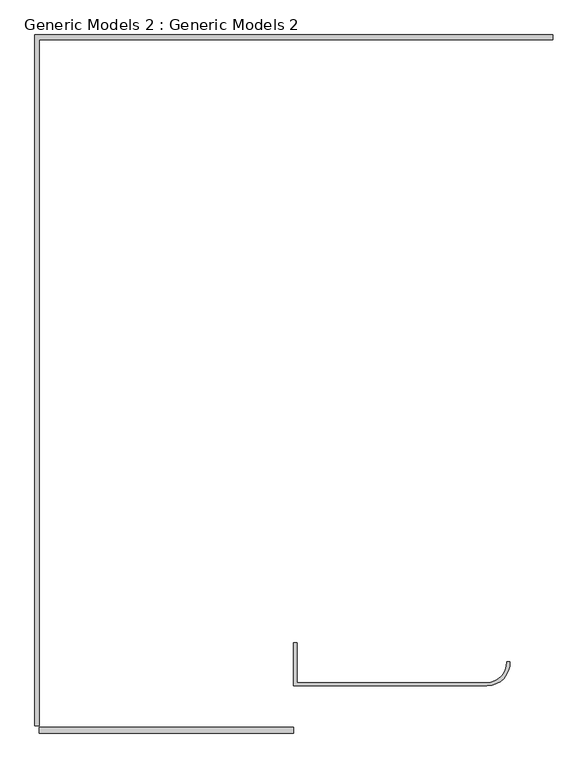
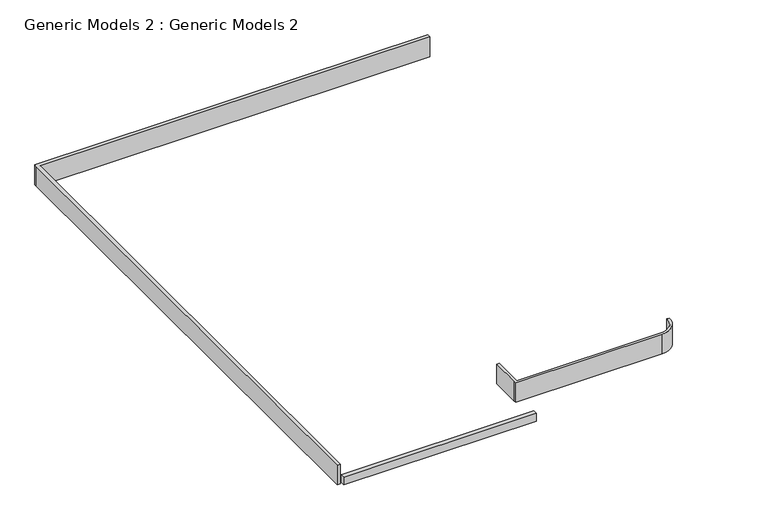
"""IFC4 building model written with IfcOpenShell, lengths in millimetres: proxy geometry, Generic Models 2 : Generic Models 2."""

from ifc_helpers import new_model, si_unit, point, frame, frame_2d, origin, origin_with_axes, place, context, project, spatial, polyline, circle_curve, trimmed, segment, composite_curve, outline, extrude, source, transform, mapped, element, save


def generic_models_2_generic_models_2_74674079(model_context):
    return source(origin(), model_context, "Body", "SweptSolid", [
        extrude(outline(polyline([(-42650.6472522, 6250.4436329), (-42650.6472522, 6059.9436329), (-51134.2472522, 6059.9436329), (-51134.2472522, 6250.4436329), (-42650.6472522, 6250.4436329)])), frame((0.0, 0.0, 91.4796875), z_axis=(0.0, 0.0, 1.0), x_axis=(1.0, 0.0, 0.0)), (0.0, 0.0, 1.0), 358.4773438),
        extrude(outline(polyline([(-33990.9791975, 29336.6093243), (-33990.9791975, 29177.2755965), (-51132.7755215, 29177.2755965), (-51132.7755215, 6297.7565956), (-51278.13478, 6297.7565956), (-51278.13478, 29257.5093141), (-51278.13478, 29336.6093243), (-33990.9791975, 29336.6093243)])), origin_with_axes(), (0.0, 0.0, 1.0), 914.4),
        extrude(outline(composite_curve([segment(trimmed(circle_curve(frame_2d((-36189.4383946, 8397.9312492)), 652.3904346), [point((-36189.4383946, 7745.5408146))], [point((-35538.4124894, 8440.1041063))], True, "CARTESIAN"), True, "CONTINUOUS"), segment(polyline([(-35538.4124894, 8440.1041063), (-35423.3146623, 8440.1041063)]), True, "CONTINUOUS"), segment(trimmed(circle_curve(frame_2d((-36189.4383946, 8410.6312492)), 766.6904346), [point((-35423.3146623, 8440.1041063))], [point((-36189.4383946, 7643.9408146))], False, "CARTESIAN"), True, "CONTINUOUS"), segment(polyline([(-36189.4383946, 7643.9408146), (-42641.0383946, 7643.9408146), (-42641.0383946, 7745.5408146), (-42641.0383946, 9075.1041063), (-42534.6852357, 9075.1041063), (-42534.6852357, 7745.5408146), (-36189.4383946, 7745.5408146)]), True, "CONTINUOUS")], self_intersect=False)), origin_with_axes(), (0.0, 0.0, 1.0), 914.4),
    ])


if __name__ == "__main__":
    model = new_model("IFC4")
    model_context = context("Model", 3, world=origin())
    ifc_project = project(units=[si_unit("LENGTHUNIT", "METRE", prefix="MILLI")], contexts=[model_context])
    site = spatial("IfcSite", under=ifc_project)
    building = spatial("IfcBuilding", under=site)
    placement = place(None, origin())
    generic_models_2_generic_models_2_shape = generic_models_2_generic_models_2_74674079(model_context)
    element("IfcBuildingElementProxy", 1, Name="Generic Models 2 : Generic Models 2", ObjectType="Generic Models 2 : Generic Models 2", at=placement, inside=building, context=model_context, shape_type="MappedRepresentation", body=[
        mapped(generic_models_2_generic_models_2_shape, transform((0.0, 0.0, 0.0), x_axis=(1.0, 0.0, 0.0), y_axis=(0.0, 1.0, 0.0), z_axis=(0.0, 0.0, 1.0))),
    ])
    save(model, "model.ifc")
